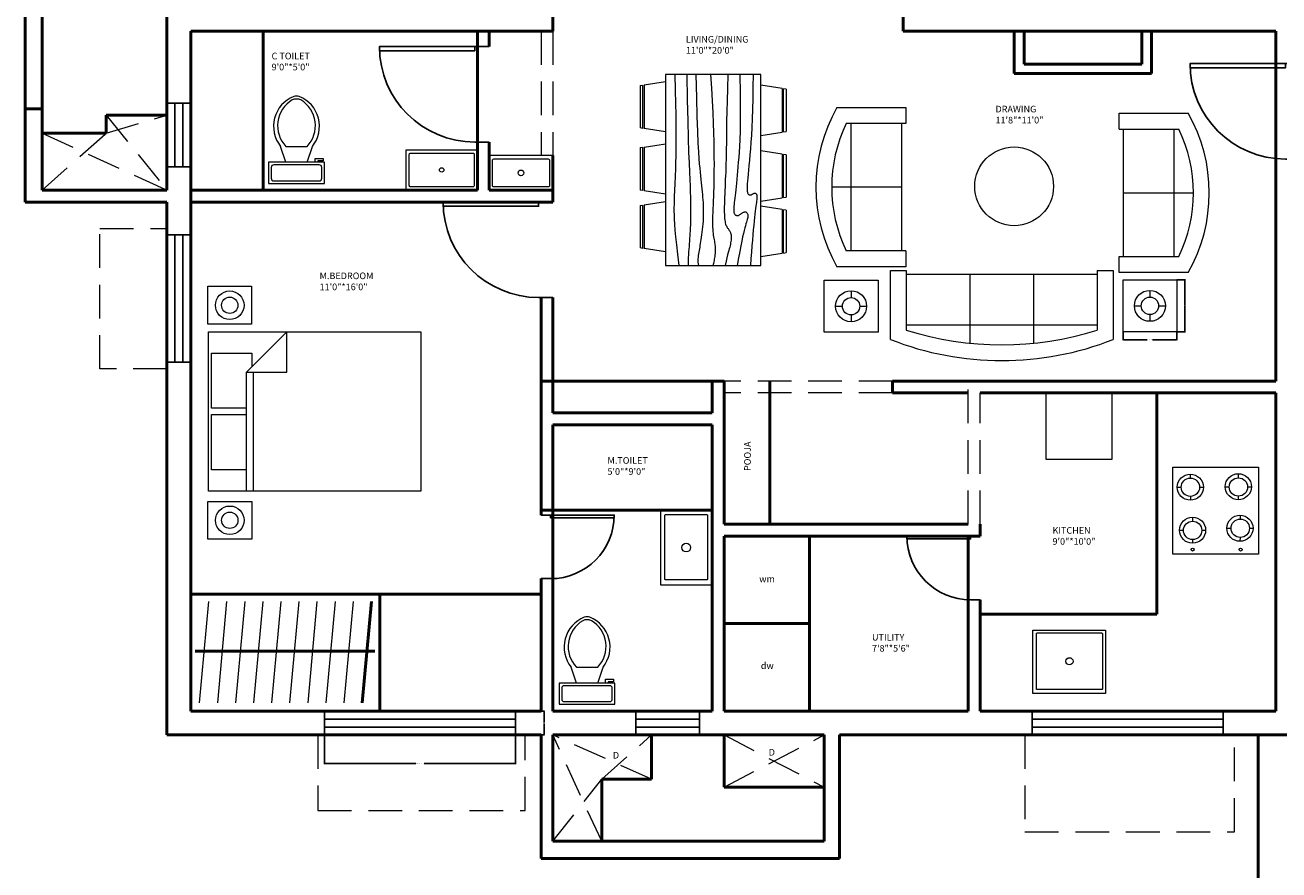
# Model space of a CAD drawing. Units: inches. Extents: x 291 to 2631, y 456 to 2623.
# Tile 14 of 22: x 1501 to 1974, y 1703 to 2022. Entities that reach past the tile are written whole.
import ezdxf

# ---------------------------------------------------------------- set-up
doc = ezdxf.new("R2010")
doc.units = ezdxf.units.IN
doc.linetypes.add('DASHED', pattern=[19.05, 12.7, -6.35])
for name, color, linetype, lineweight in [('A-ANNO-DIMS', 2, 'Continuous', 18), ('A-ANNO-TEXT', 3, 'Continuous', 25), ('A-AREA-IDEN', 7, 'Continuous', 25), ('A-DOOR', 3, 'Continuous', 25), ('A-EQPM', 8, 'Continuous', 18), ('A-FLOR-FIXT', 9, 'Continuous', 18), ('A-FLOR-OVHD', 1, 'DASHED', 18), ('A-FURN', 8, 'Continuous', 18), ('A-GLAZ', 4, 'Continuous', 25), ('A-WALL', 7, 'Continuous', 50)]:
    doc.layers.add(name, color=color, linetype=linetype, lineweight=lineweight)
doc.styles.get("Standard").update_dxf_attribs({"font": 'arial.ttf'})
doc.dimstyles.get("Standard").update_dxf_attribs({"dimtxt": 0.18, "dimasz": 0.18, "dimexe": 0.18, "dimexo": 0.0625, "dimgap": 0.09, "dimtad": 0, "dimtih": 1, "dimtoh": 1, "dimdec": 4, "dimzin": 0, "dimdsep": 46, "dimtxsty": 'Standard', "dimcen": 0.09, "dimadec": 0, "dimazin": 0, "dimtfac": 1, "dimtdec": 4, "dimtofl": 0, "dimtmove": 0, "dimatfit": 3, "dimfxl": 1, "dimtolj": 1, "dimtzin": 0, "dimarcsym": 0})

# ---------------------------------------------------------------- blocks, each defined once
blk = doc.blocks.new('*U2')
for p, q in [((0, 0), (0, -6)), ((40, 0), (40, -6))]:
    blk.add_line(p, q)
blk.add_lwpolyline([(0, 0), (0, 40), (1.75, 40), (1.75, 0)], close=True)
blk.add_arc((0, 0), 40, 0, 90)
blk = doc.blocks.new('Bed - Queen')
for p, q in [((0, -80.00003), (0, 0)), ((0, 0), (59.99999, 0)), ((59.99999, 0), (59.99999, -80.00003)), ((7.99999, -1.2), (28.79998, -1.2)), ((7.99999, -14.4), (7.99999, -1.2)), ((28.79998, -1.2), (28.79998, -14.4)), ((31.19999, -1.2), (51.99999, -1.2)), ((31.19999, -14.4), (31.19999, -1.2)), ((51.99999, -1.2), (51.99999, -16.4)), ((0, -14.4), (44.8, -14.4)), ((44.8, -16.8), (0, -16.8)), ((59.99999, -29.6), (44.8, -14.4)), ((44.8, -14.4), (44.8, -29.6)), ((51.99999, -16.4), (46.79936, -16.4)), ((44.8, -29.6), (59.99999, -29.6)), ((59.99999, -80.00003), (0, -80.00003))]:
    blk.add_line(p, q)
blk = doc.blocks.new('Toilet - top')
for p, q in [((9.5, -6), (9.5, -2)), ((-10, -8.5), (-8, -8.5)), ((-10, -9.5), (-10, -8.5)), ((-8, -8.5), (-8, -8)), ((-7, -8), (-7, -9.5)), ((-4, -8), (-6, -14)), ((4, -8), (6, -14)), ((-7, -9.5), (-10, -9.5)), ((4, -14), (-4, -14))]:
    blk.add_line(p, q)
blk.add_lwpolyline([(10.5, -8), (10.5, 0), (-10.5, 0), (-10.5, -8)], close=True)
for points in [[(-9.5, -2), (-9.5, -6)], [(8.5, -1), (-8.5, -1)], [(-8.5, -7), (8.5, -7)]]:
    blk.add_lwpolyline(points)
for centre, radius, start, end in [((-8.62, -1.88), 0.884, 81.8699, 188.1301), ((8.62, -1.88), 0.884, 351.8699, 98.1301), ((-8.62, -6.12), 0.884, 171.8699, 278.1301), ((8.62, -6.12), 0.884, 261.8699, 8.1301), ((3.52, -21.58), 12.17, 141.4691, 247.9714), ((4.2, -21.82), 11.33, 136.3677, 238.9468), ((-3.52, -21.58), 12.17, 292.0284, 38.5307), ((-4.2, -21.82), 11.33, 301.053, 43.6321), ((0, -27.88), 4, 245.7318, 294.2682), ((0, -29), 4, 254.8605, 285.1395)]:
    blk.add_arc(centre, radius, start, end)
blk = doc.blocks.new('Sofa - Roundback 7 ft.')
for p, q in [((-12.00002, -32.4421), (-12.00003, -6.5971)), ((11.99997, -32.4421), (11.99998, -6.5971)), ((-36.000027, -34), (-36.000027, -11.4696)), ((-35.999844, -13.3819), (35.9998, -13.3819)), ((35.99998, -34), (35.99998, -11.4696)), ((-36.000027, -32.4421), (35.99998, -32.4421))]:
    blk.add_line(p, q)
for points in [[(-36.000027, -34), (-42.000027, -34), (-42.000027, -8)], [(41.99998, -8), (41.99998, -34), (35.99998, -34)]]:
    blk.add_lwpolyline(points)
for centre, radius, start, end in [((0, -114.25), 114.25, 68.43141, 111.5686), ((-0.00001, -127.1968), 121.1968, 72.72033, 107.2797)]:
    blk.add_arc(centre, radius, start, end)
blk = doc.blocks.new('Sofa - Roundback Loveseat 5 ft.')
for p, q in [((0, -32.44198), (0, -5.99998)), ((-24, -33.99998), (-24, -11.46958)), ((-23.9998, -13.38178), (23.99986, -13.38178)), ((24.00004, -33.99998), (24.00004, -11.46958)), ((-24, -32.44198), (24.00004, -32.44198))]:
    blk.add_line(p, q)
for points in [[(-24, -33.99998), (-30, -33.99998), (-30, -7.99998)], [(30.00004, -7.99998), (30.00004, -33.99998), (24.00004, -33.99998)]]:
    blk.add_lwpolyline(points)
for centre, radius, start, end in [((0, -60.24998), 60.24998, 60.13715, 119.8628), ((0, -61.38438), 55.38444, 64.32083, 115.6792)]:
    blk.add_arc(centre, radius, start, end)
blk = doc.blocks.new('WIN-1800')
for p, q in [((0, 9), (72, 9)), ((0, 0), (0, 9)), ((0, 6), (72, 6)), ((72, 9), (72, 0)), ((72, 3), (0, 3)), ((72, 0), (0, 0))]:
    blk.add_line(p, q)
blk = doc.blocks.new('WIN-1200')
for p, q in [((0, 0), (0, 48)), ((0, 48), (9, 48)), ((3, 0), (3, 48)), ((6, 48), (6, 0)), ((9, 48), (9, 0)), ((9, 0), (0, 0))]:
    blk.add_line(p, q)
blk = doc.blocks.new('COOKTOP')
for p, q in [((6.54, 28.68), (6.54, 30.14)), ((24.62, 30.31), (24.62, 28.76)), ((1.62, 25.22), (3.08, 25.22)), ((10, 25.22), (11.46, 25.22)), ((19.7, 25.39), (21.21, 25.39)), ((28.13, 25.39), (29.54, 25.39)), ((6.54, 21.76), (6.54, 20.3)), ((24.62, 21.83), (24.62, 20.47)), ((25.35, 14.65), (25.34, 13.21)), ((7.38, 13.92), (7.38, 12.38)), ((20.32, 9.73), (21.89, 9.73)), ((28.81, 9.73), (30.16, 9.73)), ((2.46, 9), (3.95, 9)), ((7.38, 5.46), (7.38, 4.08)), ((10.87, 9), (12.3, 9)), ((25.26, 6.28), (25.24, 4.81))]:
    blk.add_line(p, q)
blk.add_lwpolyline([(0, 32.79), (32.25, 32.79), (32.25, 0), (0, 0)], close=True)
for centre, radius in [((6.54, 25.22), 4.92), ((6.54, 25.22), 3.46), ((24.62, 25.39), 4.92), ((24.67, 25.29), 3.46), ((25.24, 9.73), 4.92), ((7.38, 9), 4.92), ((7.41, 8.92), 3.46), ((25.35, 9.74), 3.46), ((7.38, 1.69), 0.572), ((25.5, 1.69), 0.572)]:
    blk.add_circle(centre, radius)
blk = doc.blocks.new('WIN-600')
for p, q in [((24, 9), (0, 9)), ((0, 9), (0, 0)), ((24, 6), (0, 6)), ((24, 0), (24, 9)), ((0, 3), (24, 3)), ((0, 0), (24, 0))]:
    blk.add_line(p, q)
blk = doc.blocks.new('LAMP-D')
for p, q in [((10.14, 15.61), (10.14, 13.05)), ((4.3, 9.77), (6.86, 9.77)), ((13.42, 9.77), (15.98, 9.77)), ((10.14, 6.49), (10.14, 3.93))]:
    blk.add_line(p, q)
blk.add_lwpolyline([(0, 19.54), (20.28, 19.54), (20.28, 0), (0, 0)], close=True)
for radius in [5.84, 3.28]:
    blk.add_circle((10.14, 9.77), radius)
blk = doc.blocks.new('*D22')
at = {"layer": 'A-ANNO-DIMS', "color": 0, "lineweight": -2, "transparency": 16777216}
for p, q in [((1613.85, 1754.17), (1613.85, 1743.26)), ((1685.85, 1754.17), (1685.85, 1743.26)), ((1614.03, 1743.44), (1648.3, 1743.44)), ((1685.67, 1743.44), (1651.4, 1743.44))]:
    blk.add_line(p, q, dxfattribs=at)
at = {"layer": 'A-ANNO-DIMS', "color": 0, "transparency": 16777216}
for points in [[(1614.03, 1743.47), (1614.03, 1743.41), (1613.85, 1743.44)], [(1685.67, 1743.47), (1685.67, 1743.41), (1685.85, 1743.44)]]:
    blk.add_solid(points, dxfattribs=at)
at = {"layer": 'DEFPOINTS', "color": 0, "transparency": 16777216}
for p in [(1613.85, 1754.24), (1685.85, 1754.24), (1685.85, 1743.44)]:
    blk.add_point(p, dxfattribs=at)
at = {"layer": 'A-ANNO-DIMS', "color": 0, "transparency": 16777216, "insert": (1649.85, 1743.44), "char_height": 0.18, "attachment_point": 5}
blk.add_mtext('\\A1;WINDOW W1800 72 TYP.', dxfattribs=at)
blk = doc.blocks.new('*D23')
at = {"layer": 'A-ANNO-DIMS', "color": 0, "lineweight": -2, "transparency": 16777216}
for p, q in [((1685.91, 1763.24), (1696.83, 1763.24)), ((1696.65, 1763.06), (1696.65, 1758.92)), ((1696.65, 1754.42), (1696.65, 1758.55)), ((1685.91, 1754.24), (1696.83, 1754.24))]:
    blk.add_line(p, q, dxfattribs=at)
at = {"layer": 'A-ANNO-DIMS', "color": 0, "transparency": 16777216}
for points in [[(1696.62, 1763.06), (1696.68, 1763.06), (1696.65, 1763.24)], [(1696.62, 1754.42), (1696.68, 1754.42), (1696.65, 1754.24)]]:
    blk.add_solid(points, dxfattribs=at)
at = {"layer": 'DEFPOINTS', "color": 0, "transparency": 16777216}
for p in [(1685.85, 1763.24), (1696.65, 1763.24), (1685.85, 1754.24)]:
    blk.add_point(p, dxfattribs=at)
at = {"layer": 'A-ANNO-DIMS', "color": 0, "transparency": 16777216, "insert": (1696.65, 1758.74), "char_height": 0.18, "attachment_point": 5}
blk.add_mtext('\\A1;9 TYP.', dxfattribs=at)
blk = doc.blocks.new('*D52')
at = {"layer": 'A-ANNO-DIMS', "color": 0, "lineweight": -2, "transparency": 16777216}
for p, q in [((1914.84, 1906.26), (1914.84, 1903.1)), ((1935.12, 1906.26), (1935.12, 1903.1)), ((1915.02, 1903.28), (1923.95, 1903.28)), ((1934.94, 1903.28), (1926, 1903.28))]:
    blk.add_line(p, q, dxfattribs=at)
at = {"layer": 'A-ANNO-DIMS', "color": 0, "transparency": 16777216}
for points in [[(1915.02, 1903.31), (1915.02, 1903.25), (1914.84, 1903.28)], [(1934.94, 1903.31), (1934.94, 1903.25), (1935.12, 1903.28)]]:
    blk.add_solid(points, dxfattribs=at)
at = {"layer": 'DEFPOINTS', "color": 0, "transparency": 16777216}
for p in [(1914.84, 1906.32), (1935.12, 1906.32), (1935.12, 1903.28)]:
    blk.add_point(p, dxfattribs=at)
at = {"layer": 'A-ANNO-DIMS', "color": 0, "transparency": 16777216, "insert": (1924.98, 1903.28), "char_height": 0.18, "attachment_point": 5}
blk.add_mtext('\\A1;LAMP D 20 TYP.', dxfattribs=at)
blk = doc.blocks.new('*D53')
at = {"layer": 'A-ANNO-DIMS', "color": 0, "lineweight": -2, "transparency": 16777216}
for p, q in [((1935.18, 1925.86), (1938.34, 1925.86)), ((1938.16, 1925.68), (1938.16, 1916.27)), ((1938.16, 1906.5), (1938.16, 1915.91)), ((1935.18, 1906.32), (1938.34, 1906.32))]:
    blk.add_line(p, q, dxfattribs=at)
at = {"layer": 'A-ANNO-DIMS', "color": 0, "transparency": 16777216}
for points in [[(1938.13, 1925.68), (1938.19, 1925.68), (1938.16, 1925.86)], [(1938.13, 1906.5), (1938.19, 1906.5), (1938.16, 1906.32)]]:
    blk.add_solid(points, dxfattribs=at)
at = {"layer": 'DEFPOINTS', "color": 0, "transparency": 16777216}
for p in [(1935.12, 1925.86), (1938.16, 1925.86), (1935.12, 1906.32)]:
    blk.add_point(p, dxfattribs=at)
at = {"layer": 'A-ANNO-DIMS', "color": 0, "transparency": 16777216, "insert": (1938.16, 1916.09), "char_height": 0.18, "attachment_point": 5}
blk.add_mtext('\\A1;20 TYP.', dxfattribs=at)

msp = doc.modelspace()

# ---------------------------------------------------------------- linework, layer by layer
at = {"layer": 'A-FLOR-OVHD'}
for p, q in [((1695.49, 2019.74), (1695.49, 1972.75)), ((1699.99, 2019.74), (1699.99, 1972.75)), ((1531.59, 1987.98), (1554.49, 1959.74)), ((1531.59, 1981.19), (1554.49, 1987.98)), ((1507.45, 1981.19), (1554.49, 1959.74)), ((1507.45, 1959.74), (1531.59, 1981.19)), ((1529.23, 1892.29), (1529.23, 1945.29)), ((1529.23, 1945.29), (1554.49, 1945.29)), ((1554.49, 1892.29), (1529.23, 1892.29)), ((1827.97, 1887.74), (1764.49, 1887.74)), ((1856.49, 1833.74), (1856.49, 1887.74)), ((1827.97, 1883.24), (1764.49, 1883.24)), ((1860.99, 1833.74), (1860.99, 1883.24)), ((1611.37, 1754.24), (1611.37, 1725.73)), ((1689.5, 1725.73), (1689.5, 1754.24)), ((1718.35, 1714.15), (1699.99, 1754.24)), ((1737.1, 1737.55), (1699.99, 1754.24)), ((1718.35, 1737.55), (1737.1, 1754.24)), ((1764.49, 1754.24), (1802.21, 1734.56)), ((1764.49, 1734.56), (1802.21, 1754.24)), ((1877.86, 1754.24), (1877.86, 1717.75)), ((1956.82, 1717.75), (1956.82, 1754.24)), ((1699.99, 1714.15), (1718.35, 1737.55)), ((1611.37, 1725.73), (1689.5, 1725.73)), ((1877.86, 1717.75), (1956.82, 1717.75))]:
    msp.add_line(p, q, dxfattribs=at)
at = {"layer": 'A-FURN'}
for p, q in [((1732.89, 1999.17), (1733.89, 1999.32)), ((1732.89, 1999.17), (1732.89, 1983.17)), ((1733.89, 1983.01), (1733.89, 1999.32)), ((1734.39, 1999.4), (1742.39, 2000.65)), ((1734.39, 1999.4), (1734.39, 1982.93)), ((1742.39, 2003.35), (1742.39, 1931.35)), ((1778.39, 2003.35), (1742.39, 2003.35)), ((1778.39, 1931.35), (1778.39, 2003.35)), ((1786.4, 1998.06), (1778.39, 1999.31)), ((1786.39, 1998.06), (1786.39, 1981.59)), ((1786.89, 1981.67), (1786.89, 1997.98)), ((1787.89, 1997.83), (1786.9, 1997.99)), ((1787.89, 1997.83), (1787.89, 1981.83)), ((1733.89, 1983.01), (1732.89, 1983.17)), ((1742.39, 1981.68), (1734.39, 1982.93)), ((1778.39, 1980.34), (1786.39, 1981.59)), ((1786.89, 1981.67), (1787.89, 1981.83)), ((1732.89, 1975.75), (1733.89, 1975.91)), ((1732.89, 1975.75), (1732.89, 1959.75)), ((1733.89, 1959.59), (1733.89, 1975.91)), ((1734.39, 1975.99), (1742.39, 1977.24)), ((1734.39, 1975.98), (1734.39, 1959.51)), ((1786.4, 1973.28), (1778.39, 1974.53)), ((1786.39, 1973.28), (1786.39, 1956.81)), ((1786.89, 1956.89), (1786.89, 1973.2)), ((1787.89, 1973.05), (1786.9, 1973.21)), ((1787.89, 1973.05), (1787.89, 1957.05)), ((1733.89, 1959.6), (1732.89, 1959.75)), ((1742.39, 1958.27), (1734.39, 1959.52)), ((1778.39, 1955.56), (1786.39, 1956.81)), ((1786.89, 1956.89), (1787.89, 1957.05)), ((1732.89, 1953.91), (1733.89, 1954.06)), ((1732.89, 1953.91), (1732.89, 1937.91)), ((1733.89, 1937.75), (1733.89, 1954.06)), ((1734.39, 1954.14), (1742.39, 1955.39)), ((1734.39, 1954.14), (1734.39, 1937.67)), ((1786.4, 1952.38), (1778.39, 1953.63)), ((1786.39, 1952.38), (1786.39, 1935.91)), ((1786.89, 1935.99), (1786.89, 1952.3)), ((1787.89, 1952.15), (1786.9, 1952.3)), ((1787.89, 1952.15), (1787.89, 1936.15)), ((1733.89, 1937.75), (1732.89, 1937.91)), ((1742.39, 1936.42), (1734.39, 1937.67)), ((1778.39, 1934.66), (1786.39, 1935.91)), ((1786.89, 1935.99), (1787.89, 1936.15)), ((1742.39, 1931.35), (1778.39, 1931.35)), ((1566.82, 1766.35), (1570.31, 1804.53)), ((1573.63, 1766.35), (1577.12, 1804.53)), ((1580.44, 1766.35), (1583.93, 1804.53)), ((1587.25, 1766.35), (1590.74, 1804.53)), ((1594.06, 1766.35), (1597.55, 1804.53)), ((1600.87, 1766.35), (1604.36, 1804.53)), ((1607.68, 1766.35), (1611.17, 1804.53)), ((1614.49, 1766.35), (1617.98, 1804.53)), ((1621.3, 1766.35), (1624.79, 1804.53))]:
    msp.add_line(p, q, dxfattribs=at)
for points in [[(1745.89, 2003.35), (1746.06, 1997.44), (1746.18, 1992.39), (1746.27, 1988.08), (1746.32, 1984.43), (1746.35, 1981.32), (1746.35, 1978.66), (1746.34, 1976.33), (1746.31, 1974.23), (1746.27, 1972.28), (1746.23, 1970.44), (1746.18, 1968.72), (1746.13, 1967.11), (1746.08, 1965.59), (1746.02, 1964.16), (1745.95, 1962.8), (1745.89, 1961.52), (1745.83, 1960.3), (1745.77, 1959.12), (1745.72, 1957.96), (1745.67, 1956.81), (1745.63, 1955.63), (1745.61, 1954.42), (1745.59, 1953.16), (1745.6, 1951.81), (1745.63, 1950.36), (1745.69, 1948.74), (1745.79, 1946.87), (1745.95, 1944.69), (1746.18, 1942.12), (1746.49, 1939.09), (1746.89, 1935.53), (1747.39, 1931.35)], [(1750.39, 2003.35), (1750.58, 1993.75), (1750.76, 1985.82), (1750.94, 1979.34), (1751.11, 1974.09), (1751.27, 1969.88), (1751.41, 1966.47), (1751.54, 1963.68), (1751.64, 1961.27), (1751.72, 1959.08), (1751.79, 1957.05), (1751.83, 1955.18), (1751.85, 1953.46), (1751.86, 1951.87), (1751.85, 1950.39), (1751.84, 1949.03), (1751.81, 1947.77), (1751.77, 1946.59), (1751.73, 1945.48), (1751.68, 1944.43), (1751.63, 1943.43), (1751.57, 1942.44), (1751.5, 1941.48), (1751.43, 1940.51), (1751.35, 1939.52), (1751.27, 1938.51), (1751.19, 1937.47), (1751.11, 1936.42), (1751.04, 1935.37), (1750.98, 1934.33), (1750.93, 1933.31), (1750.9, 1932.31), (1750.89, 1931.35)], [(1753.89, 2003.35), (1754.08, 1994.54), (1754.27, 1987.44), (1754.45, 1981.82), (1754.63, 1977.46), (1754.81, 1974.13), (1754.98, 1971.59), (1755.15, 1969.62), (1755.31, 1967.98), (1755.46, 1966.48), (1755.61, 1965.08), (1755.74, 1963.77), (1755.87, 1962.52), (1755.99, 1961.35), (1756.11, 1960.23), (1756.21, 1959.15), (1756.31, 1958.1), (1756.4, 1957.08), (1756.48, 1956.08), (1756.55, 1955.09), (1756.6, 1954.1), (1756.64, 1953.12), (1756.66, 1952.13), (1756.66, 1951.12), (1756.64, 1950.1), (1756.6, 1949.06), (1756.54, 1948.01), (1756.46, 1946.95), (1756.36, 1945.9), (1756.25, 1944.88), (1756.14, 1943.88), (1756.02, 1942.92), (1755.89, 1942.02), (1755.77, 1941.17), (1755.64, 1940.38), (1755.52, 1939.64), (1755.4, 1938.93), (1755.28, 1938.25), (1755.16, 1937.6), (1755.05, 1936.95), (1754.93, 1936.31), (1754.83, 1935.67), (1754.73, 1935.03), (1754.66, 1934.39), (1754.62, 1933.75), (1754.61, 1933.13), (1754.65, 1932.52), (1754.74, 1931.93), (1754.89, 1931.35)], [(1759.39, 2003.35), (1759.73, 1998.14), (1760.01, 1993.37), (1760.23, 1989), (1760.4, 1985.01), (1760.52, 1981.35), (1760.61, 1978.01), (1760.66, 1974.93), (1760.68, 1972.1), (1760.69, 1969.49), (1760.68, 1967.06), (1760.65, 1964.82), (1760.62, 1962.74), (1760.57, 1960.8), (1760.51, 1958.99), (1760.45, 1957.29), (1760.39, 1955.69), (1760.33, 1954.16), (1760.27, 1952.72), (1760.22, 1951.35), (1760.17, 1950.07), (1760.14, 1948.87), (1760.12, 1947.75), (1760.12, 1946.72), (1760.14, 1945.77), (1760.18, 1944.9), (1760.25, 1944.12), (1760.32, 1943.4), (1760.41, 1942.74), (1760.51, 1942.13), (1760.61, 1941.56), (1760.71, 1941.03), (1760.81, 1940.52), (1760.9, 1940.03), (1760.98, 1939.54), (1761.05, 1939.06), (1761.1, 1938.58), (1761.14, 1938.09), (1761.16, 1937.59), (1761.16, 1937.07), (1761.14, 1936.52), (1761.1, 1935.94), (1761.04, 1935.35), (1760.96, 1934.76), (1760.88, 1934.19), (1760.79, 1933.65), (1760.71, 1933.16), (1760.63, 1932.74), (1760.56, 1932.39), (1760.5, 1932.14), (1760.46, 1931.97), (1760.43, 1931.85), (1760.41, 1931.76), (1760.4, 1931.69), (1760.39, 1931.62), (1760.39, 1931.51), (1760.39, 1931.35)], [(1765.89, 2003.35), (1765.73, 1998.07), (1765.6, 1993.42), (1765.51, 1989.35), (1765.44, 1985.78), (1765.4, 1982.65), (1765.36, 1979.9), (1765.34, 1977.46), (1765.31, 1975.27), (1765.27, 1973.26), (1765.23, 1971.41), (1765.18, 1969.7), (1765.13, 1968.09), (1765.08, 1966.58), (1765.02, 1965.13), (1764.95, 1963.73), (1764.89, 1962.35), (1764.83, 1960.98), (1764.77, 1959.62), (1764.71, 1958.28), (1764.66, 1956.98), (1764.62, 1955.72), (1764.59, 1954.52), (1764.57, 1953.4), (1764.56, 1952.35), (1764.57, 1951.4), (1764.59, 1950.53), (1764.63, 1949.75), (1764.68, 1949.05), (1764.75, 1948.42), (1764.84, 1947.86), (1764.94, 1947.37), (1765.06, 1946.94), (1765.19, 1946.56), (1765.34, 1946.22), (1765.49, 1945.93), (1765.65, 1945.67), (1765.82, 1945.43), (1765.98, 1945.2), (1766.15, 1944.99), (1766.31, 1944.77), (1766.46, 1944.55), (1766.6, 1944.31), (1766.73, 1944.06), (1766.85, 1943.8), (1766.95, 1943.52), (1767.04, 1943.21), (1767.1, 1942.88), (1767.14, 1942.52), (1767.16, 1942.13), (1767.16, 1941.71), (1767.13, 1941.27), (1767.09, 1940.8), (1767.03, 1940.31), (1766.94, 1939.81), (1766.84, 1939.3), (1766.73, 1938.77), (1766.59, 1938.23), (1766.44, 1937.65), (1766.26, 1936.99), (1766.06, 1936.22), (1765.82, 1935.3), (1765.55, 1934.21), (1765.24, 1932.91), (1764.89, 1931.35)], [(1770.39, 2003.35), (1770.53, 1996.33), (1770.6, 1990.53), (1770.59, 1985.78), (1770.53, 1981.92), (1770.42, 1978.79), (1770.29, 1976.23), (1770.13, 1974.07), (1769.98, 1972.14), (1769.82, 1970.32), (1769.68, 1968.58), (1769.54, 1966.91), (1769.4, 1965.33), (1769.27, 1963.83), (1769.14, 1962.41), (1769.02, 1961.09), (1768.89, 1959.85), (1768.77, 1958.71), (1768.65, 1957.66), (1768.53, 1956.7), (1768.42, 1955.82), (1768.33, 1955.03), (1768.25, 1954.31), (1768.18, 1953.67), (1768.14, 1953.1), (1768.12, 1952.61), (1768.13, 1952.17), (1768.15, 1951.8), (1768.19, 1951.48), (1768.26, 1951.2), (1768.34, 1950.97), (1768.44, 1950.77), (1768.56, 1950.6), (1768.69, 1950.46), (1768.84, 1950.34), (1769, 1950.24), (1769.16, 1950.18), (1769.34, 1950.13), (1769.52, 1950.12), (1769.71, 1950.14), (1769.89, 1950.19), (1770.08, 1950.26), (1770.27, 1950.37), (1770.45, 1950.49), (1770.64, 1950.62), (1770.83, 1950.77), (1771.02, 1950.91), (1771.2, 1951.05), (1771.39, 1951.19), (1771.58, 1951.3), (1771.77, 1951.4), (1771.95, 1951.48), (1772.13, 1951.53), (1772.31, 1951.55), (1772.48, 1951.55), (1772.65, 1951.51), (1772.81, 1951.44), (1772.96, 1951.32), (1773.1, 1951.17), (1773.22, 1950.99), (1773.33, 1950.78), (1773.41, 1950.54), (1773.47, 1950.28), (1773.49, 1949.99), (1773.48, 1949.69), (1773.43, 1949.36), (1773.34, 1949.01), (1773.22, 1948.61), (1773.07, 1948.16), (1772.9, 1947.63), (1772.71, 1947.02), (1772.5, 1946.31), (1772.27, 1945.48), (1772.03, 1944.52), (1771.77, 1943.39), (1771.48, 1942.07), (1771.16, 1940.52), (1770.8, 1938.71), (1770.39, 1936.6), (1769.92, 1934.16), (1769.39, 1931.35)], [(1775.39, 2003.35), (1775.37, 1998.53), (1775.31, 1994.16), (1775.21, 1990.21), (1775.08, 1986.63), (1774.93, 1983.39), (1774.76, 1980.45), (1774.58, 1977.77), (1774.39, 1975.31), (1774.21, 1973.04), (1774.02, 1970.96), (1773.85, 1969.05), (1773.68, 1967.32), (1773.54, 1965.76), (1773.41, 1964.37), (1773.3, 1963.15), (1773.23, 1962.1), (1773.18, 1961.21), (1773.16, 1960.47), (1773.17, 1959.86), (1773.2, 1959.37), (1773.26, 1958.98), (1773.34, 1958.68), (1773.44, 1958.45), (1773.56, 1958.27), (1773.69, 1958.13), (1773.84, 1958.03), (1773.99, 1957.96), (1774.15, 1957.93), (1774.32, 1957.92), (1774.48, 1957.93), (1774.65, 1957.97), (1774.81, 1958.02), (1774.96, 1958.09), (1775.11, 1958.17), (1775.25, 1958.26), (1775.38, 1958.34), (1775.51, 1958.43), (1775.64, 1958.5), (1775.77, 1958.56), (1775.89, 1958.6), (1776.02, 1958.62), (1776.14, 1958.62), (1776.26, 1958.59), (1776.37, 1958.54), (1776.48, 1958.47), (1776.57, 1958.37), (1776.66, 1958.25), (1776.73, 1958.1), (1776.78, 1957.93), (1776.82, 1957.74), (1776.84, 1957.5), (1776.85, 1957.23), (1776.84, 1956.91), (1776.82, 1956.53), (1776.78, 1956.1), (1776.73, 1955.6), (1776.66, 1955.03), (1776.57, 1954.38), (1776.47, 1953.64), (1776.36, 1952.79), (1776.24, 1951.81), (1776.1, 1950.71), (1775.96, 1949.46), (1775.81, 1948.06), (1775.65, 1946.49), (1775.48, 1944.76), (1775.31, 1942.88), (1775.13, 1940.85), (1774.95, 1938.67), (1774.77, 1936.36), (1774.58, 1933.92), (1774.39, 1931.35)]]:
    msp.add_lwpolyline(points, dxfattribs=at)
for points in [[(1671.49, 1959.74), (1644.65, 1959.74), (1644.65, 1974.99), (1671.49, 1974.99)], [(1675.99, 1959.74), (1699.99, 1959.74), (1699.99, 1972.75), (1675.99, 1972.75)], [(1569.93, 1923.47), (1586.41, 1923.47), (1586.41, 1909.17), (1569.93, 1909.17)], [(1885.83, 1883.24), (1910.68, 1883.24), (1910.68, 1858.11), (1885.83, 1858.11)], [(1569.95, 1842.35), (1586.44, 1842.35), (1586.44, 1828.05), (1569.95, 1828.05)], [(1759.99, 1838.99), (1740.48, 1838.99), (1740.48, 1810.82), (1759.99, 1810.82)], [(1880.85, 1793.83), (1908.29, 1793.83), (1908.29, 1769.93), (1880.85, 1769.93)]]:
    msp.add_lwpolyline(points, close=True, dxfattribs=at)
for points in [[(1646.32, 1973.7), (1669.8, 1973.7, -0.414214), (1670.3, 1973.2), (1670.3, 1961.5, -0.414214), (1669.8, 1961), (1646.32, 1961, -0.414214), (1645.82, 1961.5), (1645.82, 1973.2, -0.414214)], [(1677.64, 1971.51), (1698.2, 1971.51, -0.414214), (1698.7, 1971.01), (1698.7, 1961.45, -0.414214), (1698.2, 1960.95), (1677.64, 1960.95, -0.414214), (1677.14, 1961.45), (1677.14, 1971.01, -0.414214)], [(1742.43, 1837.35), (1757.96, 1837.35, -0.414214), (1758.26, 1837.05), (1758.26, 1813.04, -0.414214), (1757.96, 1812.74), (1742.43, 1812.74, -0.414214), (1742.13, 1813.04), (1742.13, 1837.05, -0.414214)], [(1882.49, 1792.72), (1906.79, 1792.72, -0.414214), (1907.09, 1792.42), (1907.09, 1771.64, -0.414214), (1906.79, 1771.34), (1882.49, 1771.34, -0.414214), (1882.19, 1771.64), (1882.19, 1792.42, -0.414214)]]:
    msp.add_lwpolyline(points, format="xyb", close=True, dxfattribs=at)
for centre, radius in [((1873.79, 1961.16), 14.85), ((1658.06, 1967.35), 0.846), ((1687.92, 1966.23), 1.07), ((1578.17, 1916.32), 5.39), ((1578.17, 1916.32), 3.08), ((1578.19, 1835.2), 5.39), ((1578.19, 1835.2), 3.08), ((1750.24, 1824.9), 1.63), ((1894.64, 1782.03), 1.36)]:
    msp.add_circle(centre, radius, dxfattribs=at)
at = {"layer": 'A-WALL'}
for p, q in [((1501.02, 2083.8), (1501.02, 1959.74)), ((1507.45, 2078.92), (1507.45, 1959.74)), ((1554.49, 2078.92), (1554.49, 1959.74)), ((1699.99, 2027.53), (1699.99, 2019.74)), ((1831.99, 2026.78), (1831.99, 2019.74)), ((1699.99, 2019.74), (1563.49, 2019.74)), ((1563.49, 2019.74), (1563.49, 1763.24)), ((1590.75, 2019.74), (1590.75, 1959.74)), ((1671.49, 2019.74), (1671.49, 1959.74)), ((1675.99, 2019.74), (1675.99, 2013.85)), ((1972.49, 2019.74), (1831.99, 2019.74)), ((1873.79, 2019.74), (1873.79, 2003.7)), ((1877.57, 2019.74), (1877.57, 2007.24)), ((1921.97, 2007.24), (1921.97, 2019.74)), ((1925.56, 2003.7), (1925.56, 2019.74)), ((1972.49, 2019.74), (1972.49, 1887.74)), ((1877.57, 2007.24), (1921.97, 2007.24)), ((1873.79, 2003.7), (1925.56, 2003.7)), ((1501.02, 1990.44), (1507.45, 1990.44)), ((1531.59, 1981.19), (1531.59, 1987.98)), ((1531.59, 1987.98), (1554.49, 1987.98)), ((1507.45, 1981.19), (1531.59, 1981.19)), ((1675.99, 1977.85), (1675.99, 1959.74)), ((1699.99, 1972.75), (1699.99, 1955.24)), ((1501.02, 1955.24), (1501.02, 1959.74)), ((1507.45, 1959.74), (1554.49, 1959.74)), ((1671.49, 1959.74), (1563.49, 1959.74)), ((1699.99, 1959.74), (1675.99, 1959.74)), ((1554.49, 1955.24), (1501.02, 1955.24)), ((1554.49, 1955.24), (1554.49, 1754.24)), ((1699.99, 1955.24), (1563.49, 1955.24)), ((1695.49, 1919.24), (1695.49, 1837.2)), ((1699.99, 1919.24), (1699.99, 1875.74)), ((1764.49, 1887.74), (1695.49, 1887.74)), ((1759.99, 1887.74), (1759.99, 1875.74)), ((1764.49, 1887.74), (1764.49, 1833.74)), ((1781.75, 1833.74), (1781.75, 1887.74)), ((1972.49, 1887.74), (1827.97, 1887.74)), ((1827.97, 1887.74), (1827.97, 1883.24)), ((1856.49, 1883.24), (1827.97, 1883.24)), ((1972.49, 1883.24), (1860.99, 1883.24)), ((1927.65, 1799.82), (1927.65, 1883.24)), ((1972.49, 1883.24), (1972.49, 1763.24)), ((1759.99, 1875.74), (1699.99, 1875.74)), ((1759.99, 1871.24), (1699.99, 1871.24)), ((1699.99, 1871.24), (1699.99, 1763.24)), ((1759.99, 1871.24), (1759.99, 1763.24)), ((1695.49, 1838.99), (1759.99, 1838.99)), ((1856.49, 1833.74), (1764.49, 1833.74)), ((1860.99, 1833.74), (1860.99, 1829.24)), ((1860.99, 1829.24), (1764.49, 1829.24)), ((1764.49, 1829.24), (1764.49, 1763.24)), ((1796.67, 1829.24), (1796.67, 1763.24)), ((1856.49, 1829.24), (1856.49, 1763.24)), ((1695.49, 1813.2), (1695.49, 1763.24)), ((1563.49, 1807.33), (1695.49, 1807.33)), ((1634.78, 1807.33), (1634.78, 1763.24)), ((1628.11, 1766.35), (1631.6, 1804.53)), ((1860.99, 1805.24), (1860.99, 1763.24)), ((1796.67, 1796.24), (1764.49, 1796.24)), ((1860.99, 1799.82), (1927.65, 1799.82)), ((1565.18, 1785.8), (1632.88, 1785.8)), ((1695.49, 1763.24), (1563.49, 1763.24)), ((1759.99, 1763.24), (1699.99, 1763.24)), ((1856.49, 1763.24), (1764.49, 1763.24)), ((1972.49, 1763.24), (1860.99, 1763.24)), ((1695.49, 1754.24), (1554.49, 1754.24)), ((1695.49, 1754.24), (1695.49, 1707.61)), ((1699.99, 1754.24), (1699.99, 1714.15)), ((1802.21, 1754.24), (1699.99, 1754.24)), ((1737.1, 1737.55), (1737.1, 1754.24)), ((1764.49, 1754.24), (1764.49, 1734.56)), ((1802.21, 1714.15), (1802.21, 1754.24)), ((1981.49, 1754.24), (1808.01, 1754.24)), ((1808.01, 1707.61), (1808.01, 1754.24)), ((1965.72, 1754.24), (1965.72, 1458.32)), ((1718.35, 1714.15), (1718.35, 1737.55)), ((1718.35, 1737.55), (1737.1, 1737.55)), ((1764.49, 1734.56), (1802.21, 1734.56)), ((1699.99, 1714.15), (1802.21, 1714.15)), ((1695.49, 1707.61), (1808.01, 1707.61))]:
    msp.add_line(p, q, dxfattribs=at)

# ---------------------------------------------------------------- block references
at = {"layer": 'A-DOOR'}
for p, xscale, yscale, zscale, rotation in [((1670.59, 2013.85), -0.9, 0.9, 0.9, 90), ((1976.09, 2007.47), -0.9, 0.9, 0.9, 90), ((1694.59, 1955.24), -0.9, 0.9, 0.9, 90), ((1699.09, 1837.2), 0.6, 0.6, 0.6, 270), ((1857.39, 1829.24), -0.6, 0.6, 0.6, 90)]:
    msp.add_blockref('*U2', p, dxfattribs=dict(at, xscale=xscale, yscale=yscale, zscale=zscale, rotation=rotation))
at = {"layer": 'A-EQPM'}
msp.add_blockref('COOKTOP', (1933.68, 1822.48), dxfattribs=at)
at = {"layer": 'A-FLOR-FIXT', "rotation": 180}
for p in [(1603.33, 1962.22), (1712.85, 1765.83)]:
    msp.add_blockref('Toilet - top', p, dxfattribs=at)
at = {"layer": 'A-FURN'}
for name, p, rotation in [('Sofa - Roundback Loveseat 5 ft.', (1799.04, 1960.85), 90), ('Sofa - Roundback Loveseat 5 ft.', (1947.37, 1958.7), 270.0000000000006), ('Sofa - Roundback 7 ft.', (1869.16, 1895.43), 180), ('Bed - Queen', (1570.13, 1846.26), 90)]:
    msp.add_blockref(name, p, dxfattribs=dict(at, rotation=rotation))
for p in [(1802.22, 1906.18), (1914.84, 1906.32)]:
    msp.add_blockref('LAMP-D', p, dxfattribs=at)
at = {"layer": 'A-GLAZ'}
for p, rotation in [((1554.49, 1992.58), 269.9999999999988), ((1755.17, 1763.24), 180)]:
    msp.add_blockref('WIN-600', p, dxfattribs=dict(at, rotation=rotation))
for name, p in [('WIN-1200', (1554.49, 1894.86)), ('WIN-1800', (1613.85, 1754.24)), ('WIN-1800', (1880.62, 1754.24))]:
    msp.add_blockref(name, p, dxfattribs=at)

# ---------------------------------------------------------------- texts
at = {"layer": 'A-ANNO-TEXT', "char_height": 2.5, "attachment_point": 1}
for s, width, insert in [('wm', 22.1843, (1777.74, 1814.34)), ('dw', 14.3307, (1778.34, 1781.64)), ('D', 2.9815, (1781.3, 1748.98)), ('D', 3.6536, (1722.57, 1747.85))]:
    msp.add_mtext_dynamic_manual_height_columns(s, width=width, gutter_width=12.5, heights=[0], dxfattribs=dict(at, insert=insert))
at = {"layer": 'A-AREA-IDEN', "char_height": 2.5, "attachment_point": 1}
for s, width, insert in [('LIVING/DINING\\P11\'0"*20\'0"', 56.3166, (1750.09, 2017.87)), ('C TOILET\\P9\'0"*5\'0"', 32.5151, (1593.94, 2011.56)), ('DRAWING\\P11\'8"*11\'0"', 45.0769, (1866.77, 1991.55)), ('M.BEDROOM\\P11\'0"*16\'0"', 56.5526, (1612.02, 1928.66)), ('M.TOILET\\P5\'0"*9\'0"', 46.2105, (1720.53, 1859.03)), ('KITCHEN\\P9\'0"*10\'0"', 44.7481, (1888.26, 1832.65)), ('UTILITY\\P7\'8"*5\'6"', 44.0989, (1820.23, 1792.36))]:
    msp.add_mtext_dynamic_manual_height_columns(s, width=width, gutter_width=12.5, heights=[0], dxfattribs=dict(at, insert=insert))
at = {"layer": 'A-AREA-IDEN', "insert": (1772.05, 1853.81), "char_height": 2.5, "attachment_point": 1, "rotation": 90}
msp.add_mtext_dynamic_manual_height_columns('POOJA', width=13.1018, gutter_width=12.5, heights=[0], dxfattribs=at)

# ---------------------------------------------------------------- dimensions: what is measured, and where the dimension line sits
at = {"layer": 'A-ANNO-DIMS'}
for base, p1, p2, picture, middle in [((1938.16, 1925.86), (1935.12, 1906.32), (1935.12, 1925.86), '*D53', (1938.16, 1916.09)), ((1696.65, 1763.24), (1685.85, 1754.24), (1685.85, 1763.24), '*D23', (1696.65, 1758.74))]:
    dim = msp.add_linear_dim(base=base, p1=p1, p2=p2, angle=90, text='<> TYP.', dimstyle='Standard', override={"dimdec": 0, "dimlfac": 1, "dimrnd": 0, "dimzin": 0, "dimdsep": 46, "dimlunit": 2}, dxfattribs=at)
    dim.commit()
    dim.dimension.update_dxf_attribs({"geometry": picture, "text_midpoint": middle})
for base, p1, p2, text, picture, middle in [((1935.12, 1903.28), (1914.84, 1906.32), (1935.12, 1906.32), 'LAMP D <> TYP.', '*D52', (1924.98, 1903.28)), ((1685.85, 1743.44), (1613.85, 1754.24), (1685.85, 1754.24), 'WINDOW W1800 <> TYP.', '*D22', (1649.85, 1743.44))]:
    dim = msp.add_linear_dim(base=base, p1=p1, p2=p2, text=text, dimstyle='Standard', override={"dimdec": 0, "dimlfac": 1, "dimrnd": 0, "dimzin": 0, "dimdsep": 46, "dimlunit": 2}, dxfattribs=at)
    dim.commit()
    dim.dimension.update_dxf_attribs({"geometry": picture, "text_midpoint": middle})

doc.saveas('drawing.dxf')
